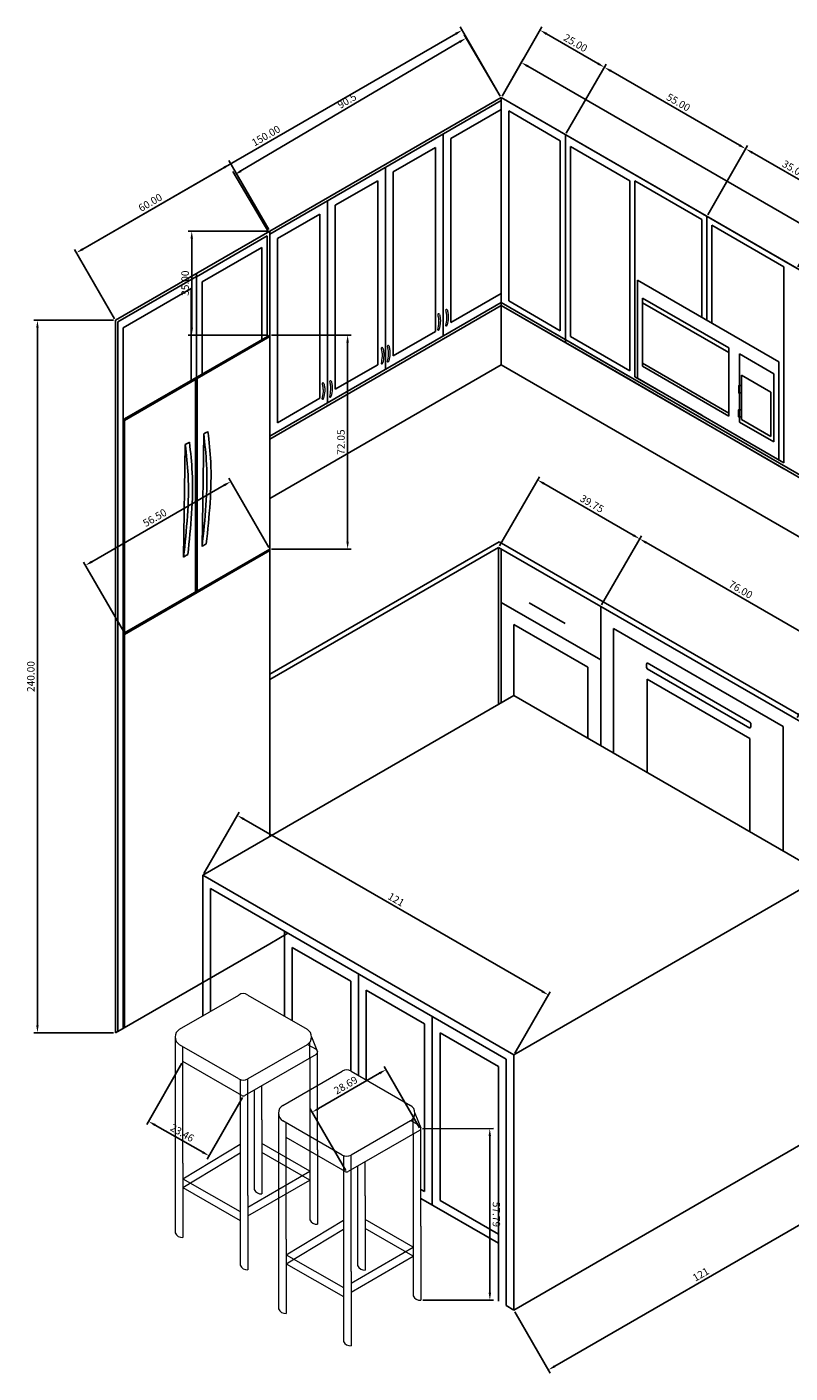
# Model space of a CAD drawing. Units: centimetres. Extents: x 21667 to 22807, y 15845 to 16565.
# Tile 1 of 4: x 21667 to 21924, y 15845 to 16298. Entities that reach past the tile are written whole.
import ezdxf

# ---------------------------------------------------------------- set-up
doc = ezdxf.new("R2010")
doc.units = ezdxf.units.CM
for name, color, linetype, lineweight in [('A-ANNO-DIMS', 2, 'Continuous', 18), ('A-ANNO-NPLT', 8, 'Continuous', 13), ('A-FURN', 8, 'Continuous', 18), ('A-FURN-CASE', 7, 'Continuous', 25), ('A-FURN-HDWR', 8, 'Continuous', 13)]:
    doc.layers.add(name, color=color, linetype=linetype, lineweight=lineweight)
doc.styles.get("Standard").update_dxf_attribs({"font": 'arial.ttf'})
doc.dimstyles.new('ISO-25', dxfattribs={"dimtxt": 2.5, "dimasz": 2.5, "dimexe": 1.25, "dimexo": 0.625, "dimtad": 1, "dimtxsty": 'Standard', "dimcen": 2.5, "dimadec": 0, "dimazin": 0, "dimtfac": 1, "dimtmove": 0, "dimatfit": 3, "dimfxl": 1, "dimarcsym": 0})

# ---------------------------------------------------------------- blocks, each defined once
blk = doc.blocks.new('*D4')
at = {"layer": 'A-ANNO-DIMS', "color": 0, "lineweight": -2, "transparency": 16777216}
for p, q in [((21827.08, 16274.89), (21834.21, 16287.25)), ((21835.75, 16284.92), (22121.54, 16119.92)), ((22117.19, 16107.39), (22124.33, 16119.75))]:
    blk.add_line(p, q, dxfattribs=at)
at = {"layer": 'A-ANNO-DIMS', "color": 0, "transparency": 16777216}
for points in [[(21835.96, 16285.28), (21835.54, 16284.56), (21833.59, 16286.17)], [(22121.75, 16120.28), (22121.33, 16119.56), (22123.71, 16118.67)]]:
    blk.add_solid(points, dxfattribs=at)
at = {"layer": 'Defpoints', "color": 0, "transparency": 16777216}
for p in [(21826.76, 16274.35), (22123.71, 16118.67), (22116.88, 16106.85)]:
    blk.add_point(p, dxfattribs=at)
at = {"layer": 'A-ANNO-DIMS', "color": 0, "transparency": 16777216, "insert": (21975.66, 16206.34), "char_height": 2.5, "attachment_point": 5, "rotation": 330}
blk.add_mtext('335', dxfattribs=at)
blk = doc.blocks.new('chair')
for p, q in [((22996.81, 16946.66), (23016.79, 16958.19)), ((23019.79, 16958.19), (23039.77, 16946.66)), ((22995.31, 16944.06), (22995.31, 16878.06)), ((23016.79, 16929.93), (22996.81, 16941.46)), ((22997.91, 16901.56), (22997.91, 16940.83)), ((23039.77, 16941.46), (23019.79, 16929.93)), ((23039.94, 16941.56), (23042.77, 16939.93)), ((23040.68, 16936.98), (23040.68, 16942.26)), ((23041.27, 16944.06), (23043.27, 16939.09)), ((23042.77, 16938.19), (23018.79, 16924.35)), ((23040.68, 16936.98), (23040.68, 16882.51)), ((23043.27, 16906.01), (23043.27, 16939.09)), ((23017.79, 16924.35), (22997.91, 16935.83)), ((23031.61, 16921.03), (23051.59, 16932.57)), ((23054.59, 16932.57), (23074.57, 16921.03)), ((23017.2, 16929.73), (23017.2, 16867.16)), ((23019.79, 16890.66), (23019.79, 16929.93)), ((23024.56, 16916.18), (23024.56, 16927.68)), ((23021.96, 16926.18), (23021.96, 16892.68)), ((23030.11, 16918.43), (23030.11, 16852.43)), ((23076.07, 16918.43), (23078.07, 16913.47)), ((23024.56, 16916.18), (23024.56, 16891.18)), ((23051.59, 16904.3), (23031.61, 16915.84)), ((23032.71, 16875.93), (23032.71, 16915.2)), ((23074.57, 16915.84), (23054.59, 16904.3)), ((23074.74, 16915.93), (23077.57, 16914.3)), ((23075.47, 16911.36), (23075.47, 16916.64)), ((23052.59, 16898.72), (23032.71, 16910.2)), ((23077.57, 16912.57), (23053.59, 16898.72)), ((23075.47, 16911.36), (23075.47, 16856.89)), ((23078.07, 16880.39), (23078.07, 16913.47)), ((22997.91, 16896.33), (23017.2, 16907.99)), ((22997.91, 16893.33), (23017.2, 16904.99)), ((23040.68, 16898.85), (23024.56, 16908.22)), ((23040.68, 16895.85), (23024.56, 16905.14)), ((23043.27, 16906.01), (23043.27, 16881.01)), ((22997.91, 16901.56), (22997.91, 16876.56)), ((23051.99, 16904.11), (23051.99, 16841.53)), ((23054.59, 16865.03), (23054.59, 16904.3)), ((23056.75, 16900.55), (23056.75, 16867.05)), ((23059.35, 16890.55), (23059.35, 16902.05)), ((22997.91, 16896.33), (23017.2, 16885.29)), ((23019.79, 16886.79), (23040.68, 16898.85)), ((23019.79, 16883.79), (23040.68, 16895.85)), ((22997.91, 16893.33), (23017.2, 16882.29)), ((23019.79, 16890.66), (23019.79, 16865.66)), ((23059.35, 16890.55), (23059.35, 16865.55)), ((23032.71, 16870.7), (23051.99, 16882.37)), ((23075.47, 16873.22), (23059.35, 16882.59)), ((23032.71, 16867.7), (23051.99, 16879.37)), ((23075.47, 16870.22), (23059.35, 16879.52)), ((23078.07, 16880.39), (23078.07, 16855.39)), ((23032.71, 16875.93), (23032.71, 16850.93)), ((23054.59, 16861.16), (23075.47, 16873.22)), ((23032.71, 16870.7), (23051.99, 16859.66)), ((23054.59, 16858.16), (23075.47, 16870.22)), ((23032.71, 16867.7), (23051.99, 16856.66)), ((23054.59, 16865.03), (23054.59, 16840.03))]:
    blk.add_line(p, q)
for centre, radius, start, end in [((23018.29, 16956.16), 2.53, 53.6213, 126.3787), ((22998.31, 16944.06), 3, 120, 240), ((23038.27, 16944.06), 3, 300, 60), ((23042.27, 16939.06), 1, 300, 60), ((23053.09, 16929.97), 3, 60, 120), ((23053.09, 16929.97), 3, 60, 120), ((23018.29, 16932.53), 3, 240, 300), ((23018.29, 16925.22), 1, 240, 300), ((23018.29, 16925.22), 1, 240, 300), ((23033.11, 16918.43), 3, 120, 240), ((23073.07, 16918.43), 3, 300, 60), ((23077.07, 16913.43), 1, 300, 60), ((23053.09, 16906.9), 3, 240, 300), ((23053.09, 16899.59), 1, 240, 300), ((23053.09, 16899.59), 1, 240, 300), ((23024.32, 16893.77), 2.6, 204.8177, 275.1823), ((23043.04, 16883.6), 2.6, 204.8177, 275.1823), ((22997.68, 16879.15), 2.6, 204.8177, 275.1823), ((23019.56, 16868.25), 2.6, 204.8177, 275.1823), ((23059.12, 16868.14), 2.6, 204.8177, 275.1823), ((23077.84, 16857.98), 2.6, 204.8177, 275.1823), ((23032.47, 16853.53), 2.6, 204.8177, 275.1823), ((23054.36, 16842.63), 2.6, 204.8177, 275.1823)]:
    blk.add_arc(centre, radius, start, end)
blk = doc.blocks.new('PULL-KNOB-B')
for centre, radius, start, end in [((0.36, 5.23), 0.305, 16.3201, 203.3621), ((0.25, 0.32), 0.321, 218.673, 1.0092)]:
    blk.add_arc(centre, radius, start, end)
for points in [[(0.08, 5.11), (0.17, 4.68), (0.36, 3.83), (0.39, 2.14), (0.16, 0.91), (0, 0.12)], [(0.65, 5.31), (0.74, 4.89), (0.94, 4.03), (0.97, 2.34), (0.73, 1.12), (0.57, 0.33)]]:
    blk.add_open_spline(points, degree=3, knots=[0, 0, 0, 0, 1.303389, 2.616446, 5.034157, 5.034157, 5.034157, 5.034157])
blk = doc.blocks.new('*D15')
at = {"layer": 'A-ANNO-DIMS', "color": 0, "lineweight": -2, "transparency": 16777216}
for p, q in [((21739.16, 16249.64), (21812.79, 16293.1)), ((21826.45, 16274.89), (21814.31, 16295.45)), ((21748.5, 16228.89), (21736.37, 16249.45))]:
    blk.add_line(p, q, dxfattribs=at)
at = {"layer": 'A-ANNO-DIMS', "color": 0, "transparency": 16777216}
for points in [[(21812.58, 16293.46), (21813.01, 16292.74), (21814.95, 16294.37)], [(21738.95, 16250), (21739.37, 16249.28), (21737, 16248.37)]]:
    blk.add_solid(points, dxfattribs=at)
at = {"layer": 'Defpoints', "color": 0, "transparency": 16777216}
for p in [(21814.95, 16294.37), (21826.76, 16274.35), (21748.82, 16228.35)]:
    blk.add_point(p, dxfattribs=at)
at = {"layer": 'A-ANNO-DIMS', "color": 0, "transparency": 16777216, "insert": (21775.01, 16273.01), "char_height": 2.5, "attachment_point": 5, "rotation": 30.5483}
blk.add_mtext('90.5', dxfattribs=at)
blk = doc.blocks.new('*D20')
at = {"layer": 'A-ANNO-DIMS', "color": 0, "lineweight": -2, "transparency": 16777216}
for p, q in [((21726.62, 16012.98), (21738.55, 16033.66)), ((21740.1, 16031.32), (21840.55, 15973.32)), ((21831.41, 15952.48), (21843.34, 15973.16))]:
    blk.add_line(p, q, dxfattribs=at)
at = {"layer": 'A-ANNO-DIMS', "color": 0, "transparency": 16777216}
for points in [[(21740.3, 16031.68), (21739.89, 16030.96), (21737.93, 16032.57)], [(21840.76, 15973.68), (21840.35, 15972.96), (21842.72, 15972.07)]]:
    blk.add_solid(points, dxfattribs=at)
at = {"layer": 'Defpoints', "color": 0, "transparency": 16777216}
for p in [(21726.3, 16012.44), (21842.72, 15972.07), (21831.09, 15951.94)]:
    blk.add_point(p, dxfattribs=at)
at = {"layer": 'A-ANNO-DIMS', "color": 0, "transparency": 16777216, "insert": (21791.26, 16003.95), "char_height": 2.5, "attachment_point": 5, "rotation": 330}
blk.add_mtext('121', dxfattribs=at)
blk = doc.blocks.new('*D21')
at = {"layer": 'A-ANNO-DIMS', "color": 0, "lineweight": -2, "transparency": 16777216}
for p, q in [((21936.2, 15925.9), (21948.13, 15905.22)), ((21945.34, 15905.05), (21844.88, 15847.05)), ((21831.41, 15865.4), (21843.34, 15844.72))]:
    blk.add_line(p, q, dxfattribs=at)
at = {"layer": 'A-ANNO-DIMS', "color": 0, "transparency": 16777216}
for points in [[(21945.13, 15905.41), (21945.55, 15904.69), (21947.51, 15906.3)], [(21844.68, 15847.41), (21845.09, 15846.69), (21842.72, 15845.8)]]:
    blk.add_solid(points, dxfattribs=at)
at = {"layer": 'Defpoints', "color": 0, "transparency": 16777216}
for p in [(21935.88, 15926.44), (21831.09, 15865.94), (21842.72, 15845.8)]:
    blk.add_point(p, dxfattribs=at)
at = {"layer": 'A-ANNO-DIMS', "color": 0, "transparency": 16777216, "insert": (21894.17, 15877.68), "char_height": 2.5, "attachment_point": 5, "rotation": 30}
blk.add_mtext('121', dxfattribs=at)
blk = doc.blocks.new('*D23')
at = {"layer": 'A-ANNO-DIMS', "color": 0, "lineweight": -2, "transparency": 16777216}
for p, q in [((21799.28, 15927.34), (21787.34, 15948.02)), ((21765.29, 15933.84), (21785.8, 15945.69)), ((21774.43, 15913), (21762.5, 15933.68))]:
    blk.add_line(p, q, dxfattribs=at)
at = {"layer": 'A-ANNO-DIMS', "color": 0, "transparency": 16777216}
for points in [[(21785.59, 15946.05), (21786.01, 15945.33), (21787.97, 15946.94)], [(21765.08, 15934.2), (21765.49, 15933.48), (21763.12, 15932.59)]]:
    blk.add_solid(points, dxfattribs=at)
at = {"layer": 'Defpoints', "color": 0, "transparency": 16777216}
for p in [(21787.97, 15946.94), (21799.59, 15926.8), (21774.75, 15912.46)]:
    blk.add_point(p, dxfattribs=at)
at = {"layer": 'A-ANNO-DIMS', "color": 0, "transparency": 16777216, "insert": (21774.59, 15941.41), "char_height": 2.5, "attachment_point": 5, "rotation": 30}
blk.add_mtext('28.69', dxfattribs=at)
blk = doc.blocks.new('*D24')
at = {"layer": 'A-ANNO-DIMS', "color": 0, "lineweight": -2, "transparency": 16777216}
for p, q in [((21719.26, 15949.15), (21707.44, 15928.41)), ((21739.64, 15937.54), (21727.82, 15916.8)), ((21726.27, 15919.12), (21710.23, 15928.26))]:
    blk.add_line(p, q, dxfattribs=at)
at = {"layer": 'A-ANNO-DIMS', "color": 0, "transparency": 16777216}
for points in [[(21710.43, 15928.62), (21710.02, 15927.9), (21708.06, 15929.5)], [(21726.47, 15919.48), (21726.06, 15918.76), (21728.44, 15917.88)]]:
    blk.add_solid(points, dxfattribs=at)
at = {"layer": 'Defpoints', "color": 0, "transparency": 16777216}
for p in [(21719.57, 15949.7), (21739.95, 15938.08), (21708.06, 15929.5)]:
    blk.add_point(p, dxfattribs=at)
at = {"layer": 'A-ANNO-DIMS', "color": 0, "transparency": 16777216, "insert": (21719.19, 15925.34), "char_height": 2.5, "attachment_point": 5, "rotation": 330.3272}
blk.add_mtext('23.46', dxfattribs=at)
blk = doc.blocks.new('*D25')
at = {"layer": 'A-ANNO-DIMS', "color": 0, "lineweight": -2, "transparency": 16777216}
for p, q in [((21800.32, 15927.04), (21824.19, 15927.06)), ((21822.94, 15924.56), (21822.97, 15871.77)), ((21800.35, 15869.25), (21824.23, 15869.27))]:
    blk.add_line(p, q, dxfattribs=at)
at = {"layer": 'A-ANNO-DIMS', "color": 0, "transparency": 16777216}
for points in [[(21823.36, 15924.56), (21822.53, 15924.56), (21822.94, 15927.06)], [(21823.39, 15871.77), (21822.56, 15871.77), (21822.98, 15869.27)]]:
    blk.add_solid(points, dxfattribs=at)
at = {"layer": 'Defpoints', "color": 0, "transparency": 16777216}
for p in [(21799.69, 15927.04), (21799.73, 15869.25), (21822.98, 15869.27)]:
    blk.add_point(p, dxfattribs=at)
at = {"layer": 'A-ANNO-DIMS', "color": 0, "transparency": 16777216, "insert": (21824.86, 15898.16), "char_height": 2.5, "attachment_point": 5, "rotation": 270.0338}
blk.add_mtext('57.79', dxfattribs=at)
blk = doc.blocks.new('*D37')
at = {"layer": 'A-ANNO-DIMS', "color": 0, "lineweight": -2, "transparency": 16777216}
for p, q in [((21696.24, 16199.35), (21669.36, 16199.35)), ((21670.61, 15961.85), (21670.61, 16196.85)), ((21696.24, 15959.35), (21669.36, 15959.35))]:
    blk.add_line(p, q, dxfattribs=at)
at = {"layer": 'A-ANNO-DIMS', "color": 0, "transparency": 16777216}
for points in [[(21670.19, 16196.85), (21671.03, 16196.85), (21670.61, 16199.35)], [(21670.19, 15961.85), (21671.03, 15961.85), (21670.61, 15959.35)]]:
    blk.add_solid(points, dxfattribs=at)
at = {"layer": 'Defpoints', "color": 0, "transparency": 16777216}
for p in [(21670.61, 16199.35), (21696.86, 16199.35), (21696.86, 15959.35)]:
    blk.add_point(p, dxfattribs=at)
at = {"layer": 'A-ANNO-DIMS', "color": 0, "transparency": 16777216, "insert": (21668.71, 16079.35), "char_height": 2.5, "attachment_point": 5, "rotation": 90}
blk.add_mtext('240.00', dxfattribs=at)
blk = doc.blocks.new('*D38')
at = {"layer": 'A-ANNO-DIMS', "color": 0, "lineweight": -2, "transparency": 16777216}
for p, q in [((21749.45, 16194.35), (21776.32, 16194.35)), ((21775.07, 16191.85), (21775.07, 16124.8)), ((21749.45, 16122.3), (21776.32, 16122.3))]:
    blk.add_line(p, q, dxfattribs=at)
at = {"layer": 'A-ANNO-DIMS', "color": 0, "transparency": 16777216}
for points in [[(21774.65, 16191.85), (21775.49, 16191.85), (21775.07, 16194.35)], [(21774.65, 16124.8), (21775.49, 16124.8), (21775.07, 16122.3)]]:
    blk.add_solid(points, dxfattribs=at)
at = {"layer": 'Defpoints', "color": 0, "transparency": 16777216}
for p in [(21748.82, 16194.35), (21748.82, 16122.3), (21775.07, 16122.3)]:
    blk.add_point(p, dxfattribs=at)
at = {"layer": 'A-ANNO-DIMS', "color": 0, "transparency": 16777216, "insert": (21773.17, 16158.32), "char_height": 2.5, "attachment_point": 5, "rotation": 90}
blk.add_mtext('72.05', dxfattribs=at)
blk = doc.blocks.new('*D39')
at = {"layer": 'A-ANNO-DIMS', "color": 0, "lineweight": -2, "transparency": 16777216}
for p, q in [((21748.2, 16229.35), (21721.32, 16229.35)), ((21722.57, 16196.85), (21722.57, 16226.85)), ((21748.2, 16194.35), (21721.32, 16194.35))]:
    blk.add_line(p, q, dxfattribs=at)
at = {"layer": 'A-ANNO-DIMS', "color": 0, "transparency": 16777216}
for points in [[(21722.15, 16226.85), (21722.99, 16226.85), (21722.57, 16229.35)], [(21722.15, 16196.85), (21722.99, 16196.85), (21722.57, 16194.35)]]:
    blk.add_solid(points, dxfattribs=at)
at = {"layer": 'Defpoints', "color": 0, "transparency": 16777216}
for p in [(21722.57, 16229.35), (21748.82, 16229.35), (21748.82, 16194.35)]:
    blk.add_point(p, dxfattribs=at)
at = {"layer": 'A-ANNO-DIMS', "color": 0, "transparency": 16777216, "insert": (21720.67, 16211.85), "char_height": 2.5, "attachment_point": 5, "rotation": 90}
blk.add_mtext('35.00', dxfattribs=at)
blk = doc.blocks.new('*D40')
at = {"layer": 'A-ANNO-DIMS', "color": 0, "lineweight": -2, "transparency": 16777216}
for p, q in [((21748.51, 16229.89), (21735.07, 16253.17)), ((21685.9, 16223.33), (21733.53, 16250.83)), ((21696.55, 16199.89), (21683.11, 16223.17))]:
    blk.add_line(p, q, dxfattribs=at)
at = {"layer": 'A-ANNO-DIMS', "color": 0, "transparency": 16777216}
for points in [[(21733.32, 16251.19), (21733.74, 16250.47), (21735.7, 16252.08)], [(21685.69, 16223.69), (21686.11, 16222.97), (21683.74, 16222.08)]]:
    blk.add_solid(points, dxfattribs=at)
at = {"layer": 'Defpoints', "color": 0, "transparency": 16777216}
for p in [(21735.7, 16252.08), (21748.82, 16229.35), (21696.86, 16199.35)]:
    blk.add_point(p, dxfattribs=at)
at = {"layer": 'A-ANNO-DIMS', "color": 0, "transparency": 16777216, "insert": (21708.77, 16238.73), "char_height": 2.5, "attachment_point": 5, "rotation": 30}
blk.add_mtext('60.00', dxfattribs=at)
blk = doc.blocks.new('*D41')
at = {"layer": 'A-ANNO-DIMS', "color": 0, "lineweight": -2, "transparency": 16777216}
for p, q in [((21826.45, 16274.89), (21813.01, 16298.17)), ((21685.9, 16223.33), (21811.47, 16295.83)), ((21696.55, 16199.89), (21683.11, 16223.17))]:
    blk.add_line(p, q, dxfattribs=at)
at = {"layer": 'A-ANNO-DIMS', "color": 0, "transparency": 16777216}
for points in [[(21811.27, 16296.19), (21811.68, 16295.47), (21813.64, 16297.08)], [(21685.69, 16223.69), (21686.11, 16222.97), (21683.74, 16222.08)]]:
    blk.add_solid(points, dxfattribs=at)
at = {"layer": 'Defpoints', "color": 0, "transparency": 16777216}
for p in [(21813.64, 16297.08), (21826.76, 16274.35), (21696.86, 16199.35)]:
    blk.add_point(p, dxfattribs=at)
at = {"layer": 'A-ANNO-DIMS', "color": 0, "transparency": 16777216, "insert": (21747.74, 16261.23), "char_height": 2.5, "attachment_point": 5, "rotation": 30}
blk.add_mtext('150.00', dxfattribs=at)
blk = doc.blocks.new('*D42')
at = {"layer": 'A-ANNO-DIMS', "color": 0, "lineweight": -2, "transparency": 16777216}
for p, q in [((21688.93, 16118.03), (21733.53, 16143.78)), ((21748.51, 16122.84), (21735.07, 16146.11)), ((21699.58, 16094.59), (21686.14, 16117.86))]:
    blk.add_line(p, q, dxfattribs=at)
at = {"layer": 'A-ANNO-DIMS', "color": 0, "transparency": 16777216}
for points in [[(21733.32, 16144.14), (21733.74, 16143.42), (21735.7, 16145.03)], [(21688.72, 16118.39), (21689.14, 16117.67), (21686.77, 16116.78)]]:
    blk.add_solid(points, dxfattribs=at)
at = {"layer": 'Defpoints', "color": 0, "transparency": 16777216}
for p in [(21735.7, 16145.03), (21748.82, 16122.3), (21699.89, 16094.05)]:
    blk.add_point(p, dxfattribs=at)
at = {"layer": 'A-ANNO-DIMS', "color": 0, "transparency": 16777216, "insert": (21710.28, 16132.55), "char_height": 2.5, "attachment_point": 5, "rotation": 30}
blk.add_mtext('56.50', dxfattribs=at)
blk = doc.blocks.new('*D43')
at = {"layer": 'A-ANNO-DIMS', "color": 0, "lineweight": -2, "transparency": 16777216}
for p, q in [((21827.08, 16274.89), (21840.51, 16298.17)), ((21842.05, 16295.83), (21859.37, 16285.83)), ((21848.73, 16262.39), (21862.16, 16285.67))]:
    blk.add_line(p, q, dxfattribs=at)
at = {"layer": 'A-ANNO-DIMS', "color": 0, "transparency": 16777216}
for points in [[(21842.26, 16296.19), (21841.85, 16295.47), (21839.89, 16297.08)], [(21859.58, 16286.19), (21859.17, 16285.47), (21861.54, 16284.58)]]:
    blk.add_solid(points, dxfattribs=at)
at = {"layer": 'Defpoints', "color": 0, "transparency": 16777216}
for p in [(21861.54, 16284.58), (21826.76, 16274.35), (21848.41, 16261.85)]:
    blk.add_point(p, dxfattribs=at)
at = {"layer": 'A-ANNO-DIMS', "color": 0, "transparency": 16777216, "insert": (21851.66, 16292.48), "char_height": 2.5, "attachment_point": 5, "rotation": 330}
blk.add_mtext('25.00', dxfattribs=at)
blk = doc.blocks.new('*D44')
at = {"layer": 'A-ANNO-DIMS', "color": 0, "lineweight": -2, "transparency": 16777216}
for p, q in [((21848.73, 16262.39), (21862.16, 16285.67)), ((21863.7, 16283.33), (21907.01, 16258.33)), ((21896.36, 16234.89), (21909.8, 16258.17))]:
    blk.add_line(p, q, dxfattribs=at)
at = {"layer": 'A-ANNO-DIMS', "color": 0, "transparency": 16777216}
for points in [[(21863.91, 16283.69), (21863.5, 16282.97), (21861.54, 16284.58)], [(21907.21, 16258.69), (21906.8, 16257.97), (21909.17, 16257.08)]]:
    blk.add_solid(points, dxfattribs=at)
at = {"layer": 'Defpoints', "color": 0, "transparency": 16777216}
for p in [(21848.41, 16261.85), (21909.17, 16257.08), (21896.05, 16234.35)]:
    blk.add_point(p, dxfattribs=at)
at = {"layer": 'A-ANNO-DIMS', "color": 0, "transparency": 16777216, "insert": (21886.31, 16272.48), "char_height": 2.5, "attachment_point": 5, "rotation": 330}
blk.add_mtext('55.00', dxfattribs=at)
blk = doc.blocks.new('*D45')
at = {"layer": 'A-ANNO-DIMS', "color": 0, "lineweight": -2, "transparency": 16777216}
for p, q in [((21896.36, 16234.89), (21909.8, 16258.17)), ((21911.34, 16255.83), (21937.32, 16240.83)), ((21926.67, 16217.39), (21940.11, 16240.67))]:
    blk.add_line(p, q, dxfattribs=at)
at = {"layer": 'A-ANNO-DIMS', "color": 0, "transparency": 16777216}
for points in [[(21911.54, 16256.19), (21911.13, 16255.47), (21909.17, 16257.08)], [(21937.53, 16241.19), (21937.11, 16240.47), (21939.48, 16239.58)]]:
    blk.add_solid(points, dxfattribs=at)
at = {"layer": 'Defpoints', "color": 0, "transparency": 16777216}
for p in [(21939.48, 16239.58), (21896.05, 16234.35), (21926.36, 16216.85)]:
    blk.add_point(p, dxfattribs=at)
at = {"layer": 'A-ANNO-DIMS', "color": 0, "transparency": 16777216, "insert": (21925.28, 16249.98), "char_height": 2.5, "attachment_point": 5, "rotation": 330}
blk.add_mtext('35.00', dxfattribs=at)
blk = doc.blocks.new('*D49')
at = {"layer": 'A-ANNO-DIMS', "color": 0, "lineweight": -2, "transparency": 16777216}
for p, q in [((21826.21, 16123.39), (21839.65, 16146.67)), ((21841.19, 16144.33), (21871.28, 16126.96)), ((21860.63, 16103.52), (21874.07, 16126.79))]:
    blk.add_line(p, q, dxfattribs=at)
at = {"layer": 'A-ANNO-DIMS', "color": 0, "transparency": 16777216}
for points in [[(21841.4, 16144.69), (21840.98, 16143.97), (21839.02, 16145.58)], [(21871.49, 16127.32), (21871.07, 16126.6), (21873.45, 16125.71)]]:
    blk.add_solid(points, dxfattribs=at)
at = {"layer": 'Defpoints', "color": 0, "transparency": 16777216}
for p in [(21873.45, 16125.71), (21825.9, 16122.85), (21860.32, 16102.97)]:
    blk.add_point(p, dxfattribs=at)
at = {"layer": 'A-ANNO-DIMS', "color": 0, "transparency": 16777216, "insert": (21857.19, 16137.29), "char_height": 2.5, "attachment_point": 5, "rotation": 330}
blk.add_mtext('39.75', dxfattribs=at)
blk = doc.blocks.new('*D50')
at = {"layer": 'A-ANNO-DIMS', "color": 0, "lineweight": -2, "transparency": 16777216}
for p, q in [((21860.63, 16103.52), (21874.07, 16126.79)), ((21875.61, 16124.46), (21937.1, 16088.96)), ((21926.45, 16065.52), (21939.89, 16088.79))]:
    blk.add_line(p, q, dxfattribs=at)
at = {"layer": 'A-ANNO-DIMS', "color": 0, "transparency": 16777216}
for points in [[(21875.82, 16124.82), (21875.4, 16124.1), (21873.45, 16125.71)], [(21937.31, 16089.32), (21936.89, 16088.6), (21939.27, 16087.71)]]:
    blk.add_solid(points, dxfattribs=at)
at = {"layer": 'Defpoints', "color": 0, "transparency": 16777216}
for p in [(21860.32, 16102.97), (21939.27, 16087.71), (21926.14, 16064.97)]:
    blk.add_point(p, dxfattribs=at)
at = {"layer": 'A-ANNO-DIMS', "color": 0, "transparency": 16777216, "insert": (21907.31, 16108.35), "char_height": 2.5, "attachment_point": 5, "rotation": 330}
blk.add_mtext('76.00', dxfattribs=at)

msp = doc.modelspace()

# ---------------------------------------------------------------- linework, layer by layer
at = {"layer": 'A-ANNO-NPLT'}
for p in [(21807.2783, 16263.0994), (21787.7927, 16251.8494), (21768.3072, 16240.5994), (21807.2783, 16193.0994), (21787.7927, 16181.8494), (21768.3072, 16170.5994), (21753.8013, 15993.563), (21778.6995, 15979.188), (21803.5977, 15964.813)]:
    msp.add_point(p, dxfattribs=at)
at = {"layer": 'A-FURN-CASE'}
for p, q in [((21826.7639, 16274.3494), (21748.8216, 16229.3494)), ((21826.7639, 16274.3494), (21826.7639, 16184.3494)), ((22116.8824, 16106.8494), (21826.7639, 16274.3494)), ((21826.7639, 16274.3494), (21826.7639, 16204.3494)), ((21826.7639, 16274.3494), (21870.0652, 16249.3494)), ((21826.7639, 16273.3494), (21748.8216, 16228.3494)), ((21826.7639, 16270.3494), (21809.8764, 16260.5994)), ((21829.362, 16269.8494), (21846.6825, 16259.8494)), ((21829.362, 16269.8494), (21829.362, 16205.8494)), ((21807.2783, 16262.0994), (21807.2783, 16194.0994)), ((21809.8764, 16260.5994), (21809.8764, 16198.5994)), ((21848.4145, 16261.8494), (21848.4145, 16191.8494)), ((21804.6802, 16257.5994), (21790.3908, 16249.3494)), ((21804.6802, 16257.5994), (21804.6802, 16195.5994)), ((21846.6825, 16259.8494), (21846.6825, 16195.8494)), ((21850.1466, 16257.8494), (21850.1466, 16193.8494)), ((21850.1466, 16257.8494), (21870.0652, 16246.3494)), ((21787.7927, 16250.8494), (21787.7927, 16182.8494)), ((21790.3908, 16249.3494), (21790.3908, 16187.3494)), ((21870.0652, 16249.3494), (21922.0267, 16219.3494)), ((21785.1947, 16246.3494), (21770.9053, 16238.0994)), ((21785.1947, 16246.3494), (21785.1947, 16184.3494)), ((21870.0652, 16246.3494), (21870.0652, 16182.3494)), ((21870.0652, 16246.3494), (21870.0652, 16182.3494)), ((21871.7972, 16246.3494), (21894.3139, 16233.3494)), ((21871.7972, 16246.3494), (21871.7972, 16180.3494)), ((21871.7972, 16246.3494), (21871.7972, 16180.3494)), ((21768.3072, 16239.5994), (21768.3072, 16171.5994)), ((21770.9053, 16238.0994), (21770.9053, 16176.0994)), ((21765.7091, 16235.0994), (21751.4197, 16226.8494)), ((21765.7091, 16235.0994), (21765.7091, 16173.0994)), ((21894.3139, 16233.3494), (21894.3139, 16200.3494)), ((21896.0459, 16234.3494), (21896.0459, 16199.3494)), ((21748.8216, 16229.3494), (21696.8601, 16199.3494)), ((21748.8216, 16229.3494), (21748.8216, 16159.3494)), ((21897.778, 16231.3494), (21897.778, 16198.3494)), ((21897.778, 16231.3494), (21922.0267, 16217.3494)), ((21724.1399, 16213.9311), (21747.9556, 16227.8435)), ((21747.9556, 16227.8435), (21747.9556, 16193.8494)), ((21751.4197, 16226.8494), (21751.4197, 16164.8494)), ((21746.2235, 16223.8494), (21726.1399, 16212.2541)), ((21746.2235, 16223.8494), (21746.2235, 16192.8494)), ((21922.0267, 16219.3494), (22116.8824, 16106.8494)), ((21922.0267, 16217.3494), (21922.0267, 16151.3494)), ((21724.1399, 16214.0994), (21697.7261, 16198.8494)), ((21724.1399, 16215.0994), (21724.1399, 16180.0994)), ((21726.1399, 16212.2541), (21726.1399, 16181.2541)), ((21872.6632, 16212.8494), (21920.2946, 16185.3494)), ((21872.6632, 16212.8494), (21920.2946, 16185.3494)), ((21872.6632, 16212.8494), (21872.6632, 16179.8494)), ((21722.4078, 16210.0994), (21699.4582, 16196.8494)), ((21722.4078, 16210.0994), (21722.4078, 16179.0994)), ((21809.8764, 16198.5994), (21826.7639, 16208.3494)), ((21874.3953, 16206.8494), (21903.4848, 16190.0546)), ((21874.3953, 16206.8494), (21903.4848, 16190.0546)), ((21874.3953, 16206.8494), (21874.3953, 16183.8494)), ((21748.8216, 16160.3494), (21826.7639, 16205.3494)), ((21748.8216, 16159.3494), (21826.7639, 16204.3494)), ((21826.7639, 16205.3494), (22116.574, 16038.0275)), ((21870.0652, 16180.3494), (21826.7639, 16205.3494)), ((21826.7639, 16204.3494), (22115.708, 16037.5275)), ((21870.0652, 16179.3494), (21826.7639, 16204.3494)), ((21846.6825, 16195.8494), (21829.362, 16205.8494)), ((21874.3953, 16205.2459), (21903.4848, 16188.4511)), ((21696.8601, 16199.3494), (21696.8601, 16019.3494)), ((21697.7261, 16198.8494), (21697.7261, 15959.8494)), ((21699.4582, 16196.8494), (21699.4582, 15960.8494)), ((21699.8912, 16166.0994), (21748.8216, 16194.3494)), ((21699.8912, 16165.5994), (21748.8216, 16193.8494)), ((21748.8216, 16159.3494), (21748.8216, 16194.3494)), ((21790.3908, 16187.3494), (21804.6802, 16195.5994)), ((21870.0652, 16182.3494), (21850.1466, 16193.8494)), ((21903.4848, 16167.0546), (21903.4848, 16190.0546)), ((21907.0047, 16165.0224), (21907.0047, 16188.0224)), ((21907.0047, 16188.0224), (21918.5626, 16181.3494)), ((21907.0047, 16188.0224), (21918.5626, 16181.3494)), ((21826.7639, 16184.3494), (21748.8216, 16139.3494)), ((21770.9053, 16176.0994), (21785.1947, 16184.3494)), ((22116.8824, 16016.8494), (21826.7639, 16184.3494)), ((21903.4848, 16168.0546), (21874.3953, 16184.8494)), ((21903.4848, 16167.0546), (21874.3953, 16183.8494)), ((21920.2946, 16185.3494), (21920.2946, 16152.3494)), ((21723.8899, 16179.5994), (21723.8899, 16107.9029)), ((21724.1399, 16179.5994), (21724.1399, 16108.0472)), ((21724.3899, 16179.5994), (21724.3899, 16108.1915)), ((21922.0267, 16149.3494), (21870.0652, 16179.3494)), ((21894.3139, 16167.3494), (21871.7972, 16180.3494)), ((21922.0267, 16151.3494), (21872.6632, 16179.8494)), ((21917.5687, 16175.1596), (21907.6834, 16180.8669)), ((21907.6834, 16180.8669), (21907.6834, 16165.954)), ((21918.5626, 16181.3494), (21918.5626, 16158.3494)), ((21917.5687, 16160.2467), (21917.5687, 16175.1596)), ((21751.4197, 16164.8494), (21765.7091, 16173.0994)), ((21699.8912, 16166.0994), (21699.8912, 15961.0994)), ((21907.6834, 16165.954), (21917.5687, 16160.2467)), ((21726.6217, 16161.1044), (21726.0633, 16123.1883)), ((21918.5626, 16158.3494), (21907.0047, 16165.0224)), ((21720.4003, 16157.5125), (21719.8419, 16119.5964)), ((21748.8216, 16160.3494), (21748.8216, 16025.438)), ((21826.0621, 16124.7546), (21748.8216, 16080.1598)), ((21961.4308, 16046.5994), (21826.0621, 16124.7546)), ((21699.8912, 16094.0472), (21748.8216, 16122.2972)), ((21699.8912, 16093.5472), (21748.8216, 16121.7972)), ((21825.8979, 16122.8494), (21748.8216, 16078.3494)), ((22064.0549, 15985.3494), (21825.8979, 16122.8494)), ((21825.8979, 16069.938), (21825.8979, 16122.8494)), ((21826.7639, 16070.438), (21826.7639, 16122.3494)), ((21860.3224, 16084.9569), (21826.7639, 16104.3319)), ((21836.1893, 16104.2101), (21848.2964, 16097.22)), ((21860.3224, 16102.9744), (21860.3224, 16056.063)), ((21860.3224, 16056.063), (21860.3224, 16102.9744)), ((21831.094, 16096.8319), (21831.094, 16072.938)), ((21855.9922, 16082.4569), (21831.094, 16096.8319)), ((21864.6525, 16095.4744), (21864.6525, 16053.563)), ((21921.8102, 16062.4744), (21864.6525, 16095.4744)), ((21910.5518, 16063.9744), (21875.9108, 16083.9744)), ((21855.9922, 16058.563), (21855.9922, 16082.4569)), ((21910.5518, 16061.9744), (21875.9108, 16081.9744)), ((21875.9108, 16078.4248), (21910.5518, 16058.4248)), ((21875.9108, 16078.4248), (21875.9108, 16047.063)), ((21831.094, 16072.938), (21726.3049, 16012.438)), ((21935.8831, 16012.438), (21831.094, 16072.938)), ((21921.8102, 16062.4744), (21921.8102, 16020.563)), ((21910.5518, 16058.4248), (21910.5518, 16027.063)), ((21696.8601, 16019.3494), (21696.8601, 15959.3494)), ((21831.094, 15951.938), (21726.3049, 16012.438)), ((21726.3049, 16012.438), (21726.3049, 15965.0522)), ((21831.094, 15951.938), (21935.8831, 16012.438)), ((21828.4959, 15950.438), (21728.903, 16007.938)), ((21728.903, 16007.938), (21728.903, 15966.5522)), ((21753.8013, 15993.563), (21753.8013, 15964.9317)), ((21748.8216, 15989.3494), (21696.8601, 15959.3494)), ((21754.9604, 15992.8937), (21748.8216, 15989.3494)), ((21756.3993, 15988.063), (21756.3993, 15963.4317)), ((21776.1014, 15976.688), (21756.3993, 15988.063)), ((21699.4582, 15978.4122), (21699.8912, 15978.6622)), ((21776.1014, 15976.688), (21776.1014, 15946.5147)), ((21778.6995, 15979.188), (21778.6995, 15945.0199)), ((21781.2976, 15973.688), (21781.2976, 15943.5199)), ((21800.9996, 15962.313), (21781.2976, 15973.688)), ((21800.9996, 15962.313), (21800.9996, 15905.8324)), ((21803.5977, 15964.813), (21803.5977, 15901.3324)), ((21825.8979, 15947.938), (21806.1958, 15959.313)), ((21806.1958, 15959.313), (21806.1958, 15902.8324)), ((21825.8979, 15868.938), (21825.8979, 15947.938)), ((21828.4959, 15867.438), (21828.4959, 15950.438)), ((21831.094, 15865.938), (21831.094, 15951.938)), ((21935.8831, 15926.438), (21831.094, 15865.938)), ((21800.9996, 15905.8324), (21799.7253, 15906.5681)), ((21825.8979, 15888.4574), (21799.7253, 15903.5681)), ((21825.8979, 15891.4574), (21806.1958, 15902.8324)), ((21828.4959, 15867.438), (21831.094, 15865.938))]:
    msp.add_line(p, q, dxfattribs=at)
for points in [[(21907.6834, 16174.8777), (21906.8135, 16174.8777), (21906.8135, 16177.3469), (21907.6834, 16177.3469)], [(21907.6834, 16166.8147), (21906.7707, 16166.8147), (21906.7707, 16169.2395), (21907.6834, 16169.2395)]]:
    msp.add_lwpolyline(points, close=True, dxfattribs=at)
for centre, radius, start, end in [((21877.921, 16082.9744), 2.2452, 153.551513, 206.448487), ((21909.2869, 16062.9744), 1.6125, 321.672285, 38.327715)]:
    msp.add_arc(centre, radius, start, end, dxfattribs=at)
for points, knots in [([(21726.6217, 16161.1044), (21726.9974, 16157.6802), (21728.3812, 16145.0699), (21727.0402, 16132.4103), (21726.0633, 16123.1883)], [0, 0, 0, 0, 10.3179718, 37.99759562, 37.99759562, 37.99759562, 37.99759562]), ([(21726.6217, 16161.1044), (21726.8982, 16161.2427), (21727.3738, 16161.4805), (21727.8432, 16161.7301), (21728.0398, 16161.8346)], [0, 0, 0, 0, 0.9273477, 1.59509938, 1.59509938, 1.59509938, 1.59509938]), ([(21728.0398, 16161.8346), (21728.4095, 16158.452), (21729.7831, 16145.8831), (21728.4454, 16133.2654), (21727.4677, 16124.0434)], [0, 0, 0, 0, 10.19230789, 37.87193171, 37.87193171, 37.87193171, 37.87193171]), ([(21720.4003, 16157.5125), (21720.776, 16154.0882), (21722.1598, 16141.478), (21720.8188, 16128.8184), (21719.8419, 16119.5964)], [0, 0, 0, 0, 10.3179718, 37.99759562, 37.99759562, 37.99759562, 37.99759562]), ([(21720.4003, 16157.5125), (21720.6768, 16157.6507), (21721.1523, 16157.8885), (21721.6218, 16158.1381), (21721.8184, 16158.2426)], [0, 0, 0, 0, 0.9273477, 1.59509938, 1.59509938, 1.59509938, 1.59509938]), ([(21721.8184, 16158.2426), (21722.188, 16154.86), (21723.5617, 16142.2911), (21722.224, 16129.6734), (21721.2463, 16120.4515)], [0, 0, 0, 0, 10.19230789, 37.87193171, 37.87193171, 37.87193171, 37.87193171]), ([(21719.8419, 16119.5964), (21720.1791, 16119.8233), (21720.6347, 16120.1299), (21721.1202, 16120.3852), (21721.2463, 16120.4515)], [0, 0, 0, 0, 1.21784744, 1.64506687, 1.64506687, 1.64506687, 1.64506687]), ([(21726.0633, 16123.1883), (21726.4006, 16123.4153), (21726.8561, 16123.7218), (21727.3416, 16123.9771), (21727.4677, 16124.0434)], [0, 0, 0, 0, 1.21784744, 1.64506687, 1.64506687, 1.64506687, 1.64506687])]:
    msp.add_open_spline(points, degree=3, knots=knots, dxfattribs=at)

# ---------------------------------------------------------------- block references
at = {"layer": 'A-FURN'}
msp.add_blockref('chair', (-1278.3451, -986.1314), dxfattribs=at)
at = {"layer": 'A-FURN-HDWR'}
for p in [(21808.03, 16197.441), (21805.3556, 16196.0119), (21786.318, 16184.6578), (21788.3806, 16185.3019), (21768.949, 16173.437), (21766.4295, 16172.7466)]:
    msp.add_blockref('PULL-KNOB-B', p, dxfattribs=at)

# ---------------------------------------------------------------- dimensions: what is measured, and where the dimension line sits
at = {"layer": 'A-ANNO-DIMS'}
for base, p1, p2, angle, override, picture, middle in [((21813.6389, 16297.0826), (21696.8601, 16199.3494), (21826.7639, 16274.3494), 30, {"dimdec": 2, "dimlfac": 1, "dimrnd": 0, "dimzin": 0, "dimdsep": 46, "dimlunit": 2}, '*D41', (21747.7363, 16261.2293)), ((21861.5395, 16284.5826), (21826.7639, 16274.3494), (21848.4145, 16261.8494), 330, {"dimdec": 2, "dimlfac": 1, "dimrnd": 0, "dimzin": 0, "dimdsep": 46, "dimlunit": 2}, '*D43', (21851.6649, 16292.4793)), ((21814.9468, 16294.3724), (21748.8216, 16228.3494), (21826.7639, 16274.3494), 30.548266, {"dimdec": 1, "dimlfac": 1, "dimrnd": 0, "dimzin": 0, "dimdsep": 46, "dimlunit": 2}, '*D15', (21775.0092, 16273.0099)), ((21909.1709, 16257.0826), (21848.4145, 16261.8494), (21896.0459, 16234.3494), 330, {"dimdec": 2, "dimlfac": 1, "dimrnd": 0, "dimzin": 0, "dimdsep": 46, "dimlunit": 2}, '*D44', (21886.3059, 16272.4793)), ((21939.4818, 16239.5826), (21896.0459, 16234.3494), (21926.3568, 16216.8494), 330, {"dimdec": 2, "dimlfac": 1, "dimrnd": 0, "dimzin": 0, "dimdsep": 46, "dimlunit": 2}, '*D45', (21925.2775, 16249.98)), ((21735.6966, 16252.0826), (21696.8601, 16199.3494), (21748.8216, 16229.3494), 30, {"dimdec": 2, "dimlfac": 1, "dimrnd": 0, "dimzin": 0, "dimdsep": 46, "dimlunit": 2}, '*D40', (21708.7651, 16238.7293)), ((21722.5716, 16229.3494), (21748.8216, 16194.3494), (21748.8216, 16229.3494), 90, {"dimdec": 2, "dimlfac": 1, "dimrnd": 0, "dimzin": 0, "dimdsep": 46, "dimlunit": 2}, '*D39', (21720.6693, 16211.8494)), ((21670.6101, 16199.3494), (21696.8601, 15959.3494), (21696.8601, 16199.3494), 90, {"dimdec": 2, "dimlfac": 1, "dimrnd": 0, "dimzin": 0, "dimdsep": 46, "dimlunit": 2}, '*D37', (21668.7086, 16079.3494)), ((21775.0716, 16122.2972), (21748.8216, 16194.3494), (21748.8216, 16122.2972), 270, {"dimdec": 2, "dimlfac": 1, "dimrnd": 0, "dimzin": 0, "dimdsep": 46, "dimlunit": 2}, '*D38', (21773.1702, 16158.3233)), ((21735.6966, 16145.0304), (21699.8912, 16094.0472), (21748.8216, 16122.2972), 30, {"dimdec": 2, "dimlfac": 1, "dimrnd": 0, "dimzin": 0, "dimdsep": 46, "dimlunit": 2}, '*D42', (21710.2807, 16132.5521)), ((21873.4474, 16125.7076), (21825.8979, 16122.8494), (21860.3224, 16102.9744), 330, {"dimdec": 2, "dimlfac": 1, "dimrnd": 0, "dimzin": 0, "dimdsep": 46, "dimlunit": 2}, '*D49', (21857.1863, 16137.2925)), ((21939.2653, 16087.7076), (21860.3224, 16102.9744), (21926.1403, 16064.9744), 330, {"dimdec": 2, "dimlfac": 1, "dimrnd": 0, "dimzin": 0, "dimdsep": 46, "dimlunit": 2}, '*D50', (21907.3071, 16108.3543)), ((21842.719, 15972.073), (21726.3049, 16012.438), (21831.094, 15951.938), 330, {"dimdec": 0, "dimlfac": 1, "dimrnd": 0, "dimzin": 0, "dimdsep": 46, "dimlunit": 2}, '*D20', (21791.2645, 16003.9513)), ((21708.0562, 15929.4963), (21739.9488, 15938.0842), (21719.5661, 15949.6974), 150.32722, {"dimdec": 2, "dimlfac": 1, "dimrnd": 0, "dimzin": 0, "dimdsep": 46, "dimlunit": 2}, '*D24', (21719.1893, 15925.3425)), ((21787.9669, 15946.938), (21774.7451, 15912.4577), (21799.5919, 15926.803), 30, {"dimdec": 2, "dimlfac": 1, "dimrnd": 0, "dimzin": 0, "dimdsep": 46, "dimlunit": 2}, '*D23', (21774.5927, 15941.4121)), ((21822.9753, 15869.2679), (21799.6912, 15927.042), (21799.7253, 15869.2542), 270.033799, {"dimdec": 2, "dimlfac": 1, "dimrnd": 0, "dimzin": 0, "dimdsep": 46, "dimlunit": 2}, '*D25', (21824.8597, 15898.1629)), ((21842.719, 15845.8029), (21935.8831, 15926.438), (21831.094, 15865.938), 210, {"dimdec": 0, "dimlfac": 1, "dimrnd": 0, "dimzin": 0, "dimdsep": 46, "dimlunit": 2}, '*D21', (21894.1735, 15877.6811))]:
    dim = msp.add_linear_dim(base=base, p1=p1, p2=p2, angle=angle, dimstyle='ISO-25', override=override, dxfattribs=at)
    dim.commit()
    dim.dimension.update_dxf_attribs({"geometry": picture, "text_midpoint": middle})
dim = msp.add_linear_dim(base=(22123.7059, 16118.668), p1=(21826.7639, 16274.3494), p2=(22116.8824, 16106.8494), angle=330, dimstyle='ISO-25', override={"dimclrd": 0, "dimclre": 0, "dimclrt": 0}, dxfattribs=at)
dim.commit()
dim.dimension.update_dxf_attribs({"geometry": '*D4', "text_midpoint": (21974.7095, 16204.6911), "dimtype": 161})

doc.saveas('drawing.dxf')
